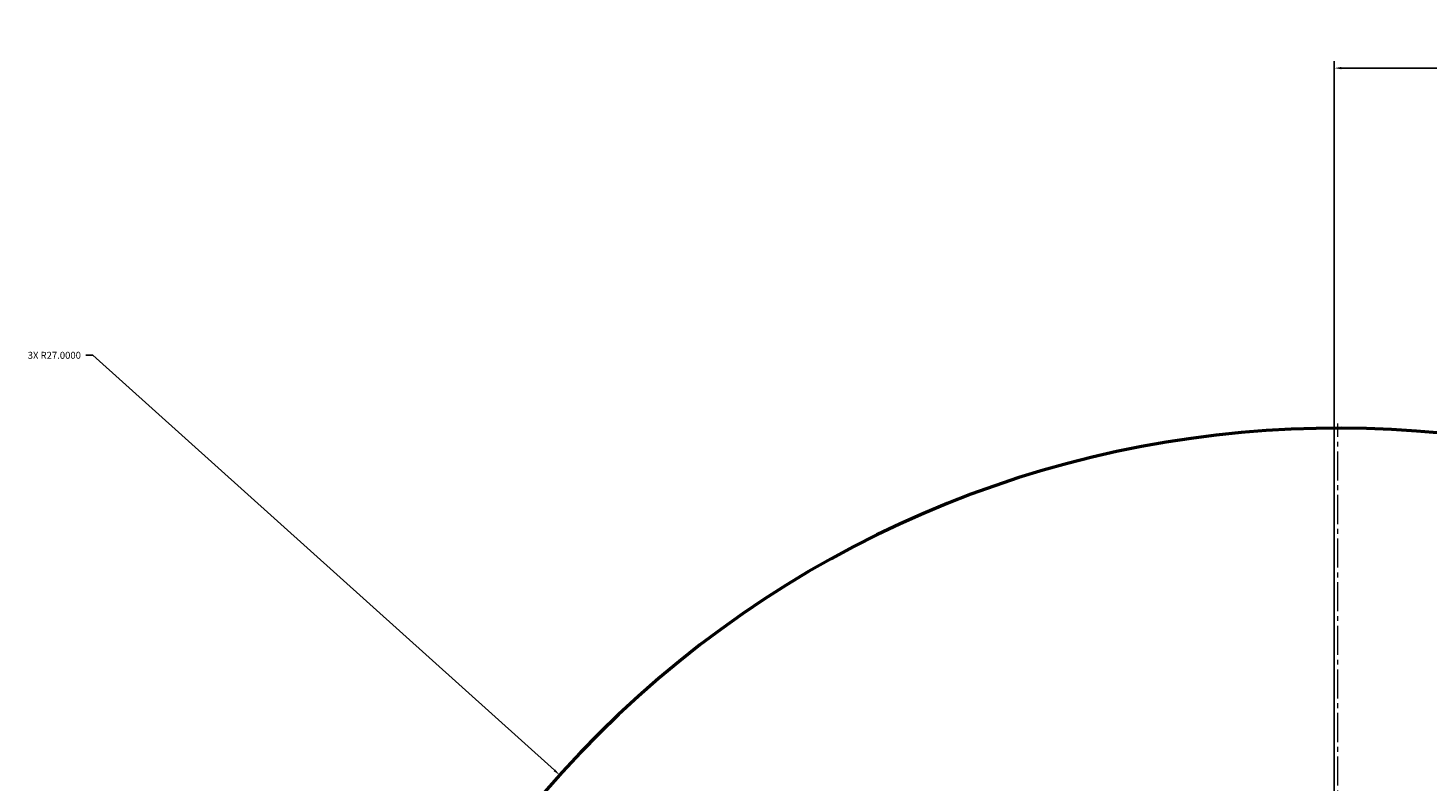
# Model space of a CAD drawing. Units: millimetres. Extents: x -60 to 113, y -37 to 126.
# Tile 14 of 17: x -23 to 13, y 106 to 126. Entities that reach past the tile are written whole.
import ezdxf

# ---------------------------------------------------------------- set-up
doc = ezdxf.new("R2010")
doc.units = ezdxf.units.MM
doc.header["$MEASUREMENT"] = 0
doc.linetypes.add('CENTER2', pattern=[1.125, 0.75, -0.125, 0.125, -0.125])
for name, color, linetype, lineweight in [('M-CNTR', 4, 'CENTER2', 18), ('M-DIMS', 2, 'Continuous', 25), ('M-OUTL', 7, 'Continuous', 50)]:
    doc.layers.add(name, color=color, linetype=linetype, lineweight=lineweight)
doc.styles.get("Standard").update_dxf_attribs({"font": 'arial.ttf'})
doc.dimstyles.get("Standard").update_dxf_attribs({"dimtxt": 0.18, "dimasz": 0.18, "dimexe": 0.18, "dimexo": 0.0625, "dimgap": 0.09, "dimtad": 0, "dimtih": 1, "dimtoh": 1, "dimdec": 4, "dimzin": 0, "dimdsep": 46, "dimtxsty": 'Standard', "dimcen": 0.09, "dimadec": 0, "dimazin": 0, "dimtfac": 1, "dimtdec": 4, "dimtofl": 0, "dimtmove": 0, "dimatfit": 3, "dimfxl": 1, "dimtolj": 1, "dimtzin": 0, "dimarcsym": 0})

# ---------------------------------------------------------------- blocks, each defined once
blk = doc.blocks.new('*U1')
at = {"layer": 'M-CNTR', "color": 0, "transparency": 16777216}
blk.add_line((0, 5.4), (0, 27.12), dxfattribs=at)
blk = doc.blocks.new('*D8')
at = {"layer": 'Defpoints', "color": 0, "transparency": 16777216}
for p in [(23.977, 96.423), (-0.678, 83.151)]:
    blk.add_point(p, dxfattribs=at)
at = {"layer": 'M-DIMS', "color": 0, "lineweight": -2, "transparency": 16777216}
for p, q in [((48.912, 109.846), (24.135, 96.508)), ((49.092, 109.846), (48.912, 109.846)), ((11.559, 89.787), (11.739, 89.787)), ((11.649, 89.697), (11.649, 89.877))]:
    blk.add_line(p, q, dxfattribs=at)
at = {"layer": 'M-DIMS', "color": 0, "transparency": 16777216}
blk.add_solid([(24.121, 96.535), (24.149, 96.482), (23.977, 96.423)], dxfattribs=at)
at = {"layer": 'M-DIMS', "color": 0, "transparency": 16777216, "insert": (51.704, 109.846), "char_height": 0.18, "attachment_point": 5}
blk.add_mtext('\\A1;{\\H11.11111x;%%C28}', dxfattribs=at)
blk = doc.blocks.new('*D17')
at = {"layer": 'Defpoints', "color": 0, "transparency": 16777216}
for p in [(67.355, 124.823), (10.532, 88.533), (67.355, 6.442)]:
    blk.add_point(p, dxfattribs=at)
at = {"layer": 'M-DIMS', "color": 0, "lineweight": -2, "transparency": 16777216}
for p, q in [((10.532, 88.595), (10.532, 125.003)), ((10.712, 124.823), (37.422, 124.823)), ((67.175, 124.823), (40.465, 124.823)), ((67.355, 6.504), (67.355, 125.003))]:
    blk.add_line(p, q, dxfattribs=at)
at = {"layer": 'M-DIMS', "color": 0, "transparency": 16777216}
for points in [[(10.712, 124.853), (10.712, 124.793), (10.532, 124.823)], [(67.175, 124.853), (67.175, 124.793), (67.355, 124.823)]]:
    blk.add_solid(points, dxfattribs=at)
at = {"layer": 'M-DIMS', "color": 0, "transparency": 16777216, "insert": (38.944, 124.823), "char_height": 0.18, "attachment_point": 5}
blk.add_mtext('\\A1;{\\H11.11111x;56}', dxfattribs=at)
blk = doc.blocks.new('*D20')
at = {"layer": 'Defpoints', "color": 0, "transparency": 16777216}
for p in [(-9.458, 106.582), (10.622, 88.533)]:
    blk.add_point(p, dxfattribs=at)
at = {"layer": 'M-DIMS', "color": 0, "lineweight": -2, "transparency": 16777216}
for p, q in [((-21.686, 117.412), (-21.506, 117.412)), ((-21.506, 117.412), (-9.592, 106.703)), ((10.532, 88.533), (10.712, 88.533)), ((10.622, 88.443), (10.622, 88.623))]:
    blk.add_line(p, q, dxfattribs=at)
at = {"layer": 'M-DIMS', "color": 0, "transparency": 16777216}
blk.add_solid([(-9.572, 106.725), (-9.612, 106.68), (-9.458, 106.582)], dxfattribs=at)
at = {"layer": 'M-DIMS', "color": 0, "transparency": 16777216, "insert": (-22.499, 117.412), "char_height": 0.18, "attachment_point": 5}
blk.add_mtext('\\A1;3X R27.0000', dxfattribs=at)

msp = doc.modelspace()

# ---------------------------------------------------------------- linework, layer by layer
at = {"layer": 'M-OUTL'}
msp.add_arc((10.62227, 88.53289), 27, 43.425324, 223.425324, dxfattribs=at)

# ---------------------------------------------------------------- block references
at = {"layer": 'M-CNTR'}
msp.add_blockref('*U1', (10.62227, 88.53289), dxfattribs=at)

# ---------------------------------------------------------------- dimensions: what is measured, and where the dimension line sits
at = {"layer": 'M-DIMS'}
dim = msp.add_linear_dim(base=(67.35481, 124.82251), p1=(10.53227, 88.53289), p2=(67.35481, 6.44179), text='{\\H11.11111x;56}', dimstyle='Standard', override={"dimclrd": 0, "dimclre": 0, "dimclrt": 0}, dxfattribs=at)
dim.commit()
dim.dimension.update_dxf_attribs({"geometry": '*D17', "text_midpoint": (38.94354, 124.82251)})
dim = msp.add_radius_dim(center=(10.62227, 88.53289), mpoint=(-9.45794, 106.58241), text='3X <>', dimstyle='Standard', override={"dimdec": 4, "dimlfac": 1, "dimrnd": 0, "dimzin": 0, "dimdsep": 46, "dimlunit": 2}, dxfattribs=at)
dim.commit()
dim.dimension.update_dxf_attribs({"geometry": '*D20', "text_midpoint": (-22.49876, 117.41213), "dimtype": 164})
dim = msp.add_diameter_dim_2p(p1=(-0.67791, 83.1508), p2=(23.97668, 96.423), text='{\\H11.11111x;%%C28}', dimstyle='Standard', override={"dimclrd": 0, "dimclre": 0, "dimclrt": 0}, dxfattribs=at)
dim.commit()
dim.dimension.update_dxf_attribs({"geometry": '*D8', "text_midpoint": (51.70419, 109.84614), "dimtype": 163})

doc.saveas('drawing.dxf')
